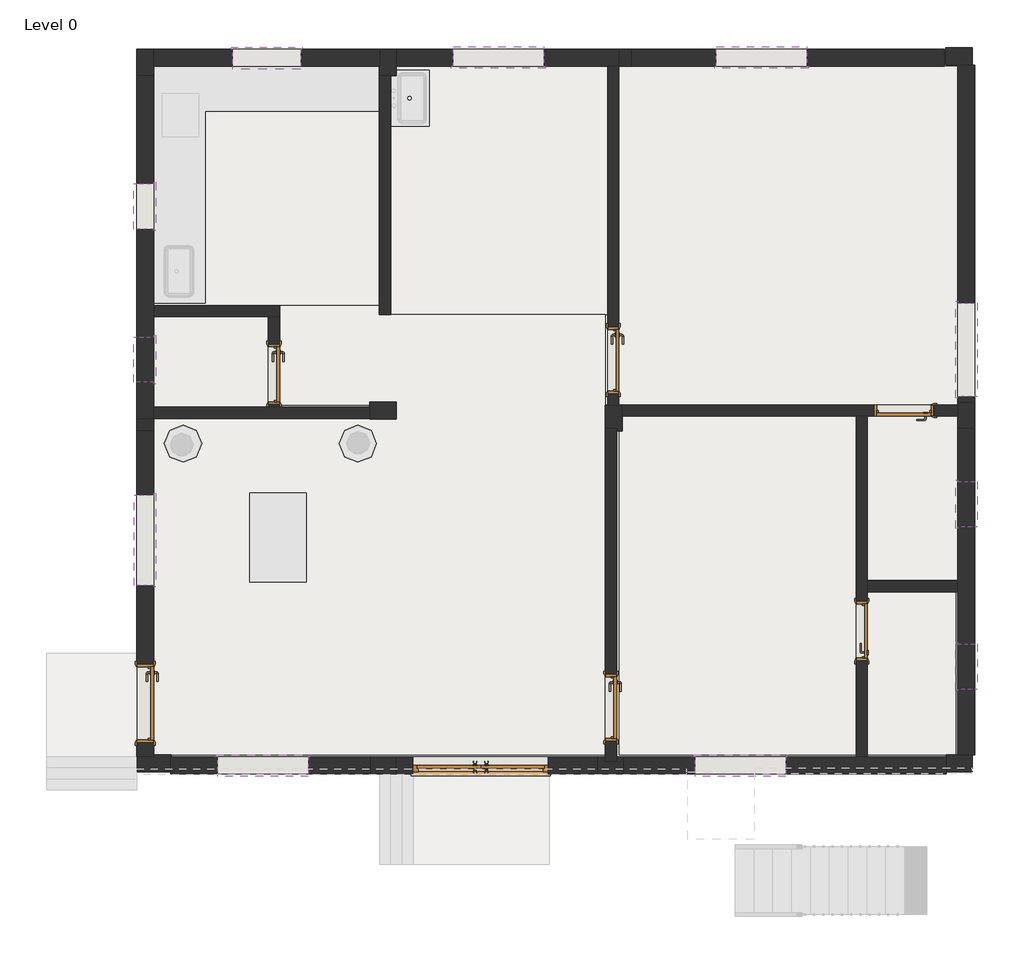
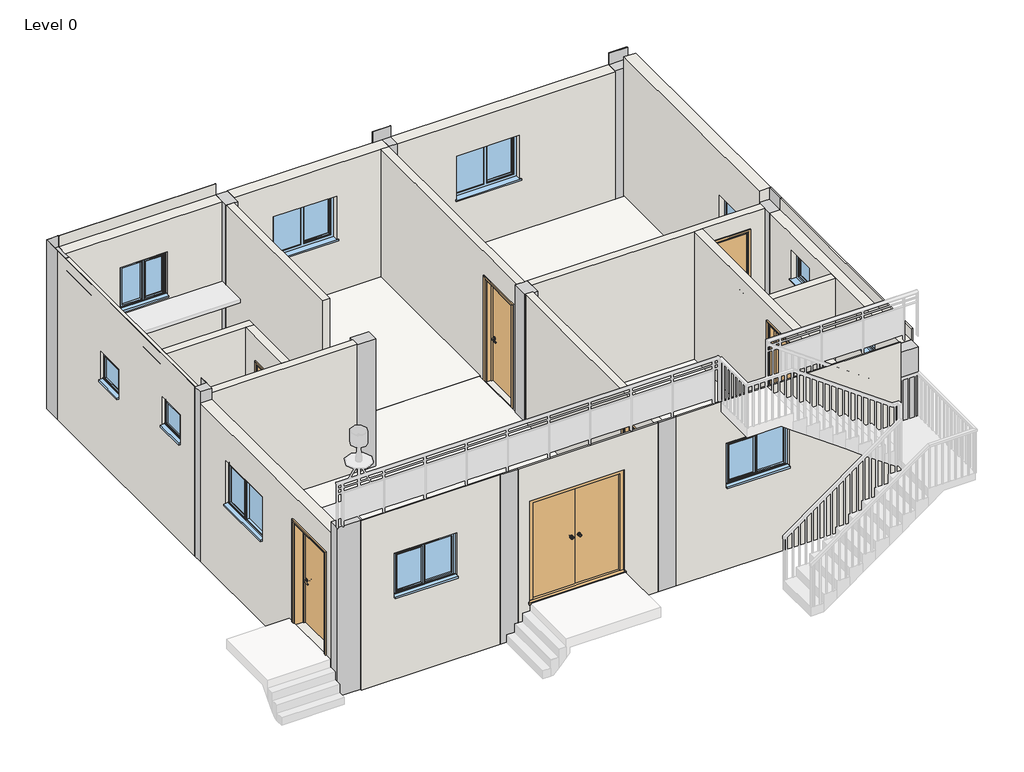
# One storey, part 1 of 3: 19 walls, 12 columns, 11 windows, 7 doors, 5 slabs.
"""IFC4 building model written with IfcOpenShell, lengths in millimetres."""

from ifc_helpers import new_model, si_unit, frame, origin, origin_with_axes, place, context, project, spatial, polyline, outline, extrude, faceted_brep, transform, mapped, element, save
from components import doors_extdbl_flush_d1_7bcd4abb, doors_intsgl_d2_1027b9ee, doors_intsgl_d3_6b78dd6f, doors_intsgl_d4_c85c0d06, doors_intsgl_d5_996c1a6b, doors_intsgl_d7_212e1d6e, windows_dbl_plain_w1_9e0d93ab, windows_dbl_plain_w3_a138f75b, windows_dbl_plain_w5_c0a8d941, windows_dbl_plain_w6_14064f4c, windows_sgl_plain_vw1_399019d4

model = new_model("IFC4")

# Units and contexts
model_context = context("Model", 3, world=origin())
ifc_project = project(units=[si_unit("LENGTHUNIT", "METRE", prefix="MILLI")], contexts=[model_context])

# Site, building, storey
site = spatial("IfcSite", under=ifc_project)
building = spatial("IfcBuilding", under=site)
storey = spatial("IfcBuildingStorey", under=building, Name="Level 0", Elevation=0.0)

# Columns
placement = place(None, origin())
element("IfcColumn", 1, ObjectType="Columns_Rectangular : C1", at=placement, inside=storey, context=model_context, shape_type="Brep", body=[
    faceted_brep([(-10027.7206387, 8256.6134098, 3000.0), (-10256.3206387, 8256.6134098, 3000.0), (-10256.3206387, 7900.9118098, 3000.0), (-10252.3493191, 7900.9118098, 3000.0), (-10252.3493191, 8254.493892, 3000.0), (-10027.7206387, 8254.493892, 3000.0), (-10027.7206387, 8256.6134098, -472.7448), (-10027.7206387, 7900.9118098, -472.7448), (-10256.3206387, 7900.9118098, -472.7448), (-10256.3206387, 8256.6134098, -472.7448), (-10027.7206387, 7900.9118098, 2769.876), (-10252.3493191, 7900.9118098, 2769.876), (-10027.7206387, 8254.493892, 2769.876), (-10252.3493191, 8254.493892, 2769.876)], [[[0, 1, 2, 3, 4, 5]], [[6, 7, 8, 9]], [[1, 0, 6, 9]], [[2, 1, 9, 8]], [[8, 7, 10, 11, 3, 2]], [[7, 6, 0, 5, 12, 10]], [[12, 13, 11, 10]], [[13, 4, 3, 11]], [[4, 13, 12, 5]]]),
])
element("IfcColumn", 2, ObjectType="Columns_Rectangular : C1", at=placement, inside=storey, context=model_context, shape_type="Brep", body=[
    faceted_brep([(-10253.9826298, 3098.473262, 3000.0), (-10025.3826298, 3098.473262, 3000.0), (-10025.3826298, 3454.174862, 3000.0), (-10025.6874298, 3454.174862, 3000.0), (-10025.6874298, 3271.6004551, 3000.0), (-10252.3493191, 3271.6004551, 3000.0), (-10253.9826298, 3271.6004551, 3000.0), (-10025.3826298, 3454.174862, -472.7448), (-10025.3826298, 3098.473262, -472.7448), (-10253.9826298, 3098.473262, -472.7448), (-10253.9826298, 3271.6004551, -472.7448), (-10025.6874298, 3271.6004551, -472.7448), (-10025.6874298, 3454.174862, -472.7448), (-10025.6874298, 3271.6004551, 2769.876)], [[[0, 1, 2, 3, 4, 5, 6]], [[7, 8, 9, 10, 11, 12]], [[2, 7, 12, 3]], [[9, 0, 6, 10]], [[1, 0, 9, 8]], [[2, 1, 8, 7]], [[11, 13, 4, 3, 12]], [[4, 13, 11, 10, 6, 5]]]),
])
element("IfcColumn", 3, ObjectType="Columns_Rectangular : C1", at=placement, inside=storey, context=model_context, shape_type="SweptSolid", body=[
    extrude(outline(polyline([(-6752.3914732, 8254.4587286), (-6752.3914732, 7898.7571286), (-6980.9914732, 7898.7571286), (-6980.9914732, 8026.4804551), (-6975.3482492, 8026.4804551), (-6975.3482492, 8254.4587286), (-6752.3914732, 8254.4587286)])), frame((0.0, 0.0, -472.7448), z_axis=(0.0, 0.0, 1.0), x_axis=(1.0, 0.0, 0.0)), (0.0, 0.0, 1.0), 3242.6208),
])
element("IfcColumn", 4, ObjectType="Columns_Rectangular : C1", at=placement, inside=storey, context=model_context, shape_type="Brep", body=[
    faceted_brep([(-3575.083968, 8257.5084176, 3000.0), (-3930.785568, 8257.5084176, 3000.0), (-3930.785568, 8254.493892, 3000.0), (-3575.083968, 8254.493892, 3000.0), (-3930.785568, 8257.5084176, -472.7448), (-3575.083968, 8257.5084176, -472.7448), (-3575.083968, 8028.9084176, -472.7448), (-3746.8074298, 8028.9084176, -472.7448), (-3746.8074298, 8254.493892, -472.7448), (-3930.785568, 8254.493892, -472.7448), (-3575.083968, 8028.9084176, 2769.876), (-3746.8074298, 8028.9084176, 2769.876), (-3575.083968, 8254.493892, 2769.876), (-3746.8074298, 8254.493892, 2769.876)], [[[0, 1, 2, 3]], [[4, 5, 6, 7, 8, 9]], [[1, 4, 9, 2]], [[7, 6, 10, 11]], [[6, 5, 0, 3, 12, 10]], [[1, 0, 5, 4]], [[9, 8, 13, 12, 3, 2]], [[8, 7, 11, 13]], [[12, 13, 11, 10]]]),
])
element("IfcColumn", 5, ObjectType="Columns_Rectangular : C1", at=placement, inside=storey, context=model_context, shape_type="SweptSolid", body=[
    extrude(outline(polyline([(8277.857647, -472.7448), (8049.257647, -472.7448), (8049.257647, 2769.876), (8254.493892, 2769.876), (8254.493892, 3000.0), (8277.857647, 3000.0), (8277.857647, -472.7448)])), frame((665.5777613, 0.0, 0.0), z_axis=(1.0, 0.0, 0.0), x_axis=(0.0, 1.0, 0.0)), (0.0, 0.0, 1.0), 355.7016),
])
element("IfcColumn", 6, ObjectType="Columns_Rectangular : C1", at=placement, inside=storey, context=model_context, shape_type="Brep", body=[
    faceted_brep([(1055.8403741, 3136.494399, 3000.0), (1055.8403741, 3492.195999, 3000.0), (1025.0682817, 3492.195999, 3000.0), (1025.0682817, 3136.494399, 3000.0), (827.2403741, 3136.494399, -472.7448), (827.2403741, 3492.195999, -472.7448), (1055.8403741, 3492.195999, -472.7448), (1055.8403741, 3136.494399, -472.7448), (1025.0682817, 3136.494399, 2769.876), (827.2403741, 3136.494399, 2769.876), (827.2403741, 3492.195999, 2769.876), (1025.0682817, 3492.195999, 2769.876), (827.2403741, 3301.5242383, 2769.876), (827.2403741, 3453.9242383, 2769.876)], [[[0, 1, 2, 3]], [[4, 5, 6, 7]], [[4, 7, 0, 3, 8, 9]], [[1, 0, 7, 6]], [[6, 5, 10, 11, 2, 1]], [[5, 4, 9, 12, 13, 10]], [[8, 11, 10, 13, 12, 9]], [[11, 8, 3, 2]]]),
])
element("IfcColumn", 7, ObjectType="Columns_Rectangular : C1", at=placement, inside=storey, context=model_context, shape_type="SweptSolid", body=[
    extrude(outline(polyline([(1025.2206817, -1501.142353), (669.5190817, -1501.142353), (669.5190817, -1272.542353), (1025.2206817, -1272.542353), (1025.2206817, -1501.142353)])), frame((0.0, 0.0, -472.7448), z_axis=(0.0, 0.0, 1.0), x_axis=(1.0, 0.0, 0.0)), (0.0, 0.0, 1.0), 3242.6208),
])
element("IfcColumn", 8, ObjectType="Columns_Rectangular : C1", at=placement, inside=storey, context=model_context, shape_type="SweptSolid", body=[
    extrude(outline(polyline([(-7108.0422732, 3492.122462), (-6752.3406732, 3492.122462), (-6752.3406732, 3263.522462), (-7108.0422732, 3263.522462), (-7108.0422732, 3492.122462)])), frame((0.0, 0.0, -472.7448), z_axis=(0.0, 0.0, 1.0), x_axis=(1.0, 0.0, 0.0)), (0.0, 0.0, 1.0), 3242.6208),
])
element("IfcColumn", 9, ObjectType="Columns_Rectangular : C1", at=placement, inside=storey, context=model_context, shape_type="Brep", body=[
    faceted_brep([(-3930.3270396, 3098.192292, -472.7448), (-3930.3270396, 3453.893892, -472.7448), (-3701.7270396, 3453.893892, -472.7448), (-3701.7270396, 3098.192292, -472.7448), (-3701.7270396, 3098.192292, 2769.876), (-3775.2396259, 3098.192292, 2769.876), (-3775.2396259, 3098.192292, 0.0), (-3927.6396259, 3098.192292, 0.0), (-3927.6396259, 3098.192292, 2769.876), (-3930.3270396, 3098.192292, 2769.876), (-3701.7270396, 3453.893892, 2769.876), (-3930.3270396, 3453.893892, 2769.876), (-3927.6396259, 3136.1864821, 2769.876), (-3775.2396259, 3136.1864821, 2769.876), (-3775.2396259, 3136.1864821, 0.0), (-3927.6396259, 3136.1864821, 0.0)], [[[0, 1, 2, 3]], [[0, 3, 4, 5, 6, 7, 8, 9]], [[3, 2, 10, 4]], [[2, 1, 11, 10]], [[1, 0, 9, 11]], [[4, 10, 11, 9, 8, 12, 13, 5]], [[13, 14, 6, 5]], [[15, 12, 8, 7]], [[14, 15, 7, 6]], [[15, 14, 13, 12]]]),
])
element("IfcColumn", 10, ObjectType="Columns_Rectangular : C2", at=placement, inside=storey, context=model_context, shape_type="Brep", body=[
    faceted_brep([(-3680.0785183, -1501.447153, 3000.0), (-4036.4886614, -1501.447153, 3000.0), (-4036.4886614, -1528.9995449, 3000.0), (-3680.0785183, -1528.9995449, 3000.0), (-4036.4886614, -1528.9995449, -472.7448), (-4036.4886614, -1300.3995449, -472.7448), (-3634.7077872, -1300.3995449, -472.7448), (-3634.7077872, -1300.9557617, -472.7448), (-3680.0785183, -1300.9557617, -472.7448), (-3680.0785183, -1528.9995449, -472.7448), (-3634.7077872, -1300.3995449, 2769.876), (-3634.7077872, -1300.9557617, 2769.876), (-4036.4886614, -1300.3995449, 2769.876), (-3927.6396259, -1300.3995449, 2769.876), (-3927.6396259, -1300.3995449, 0.0), (-3775.2396259, -1300.3995449, 0.0), (-3775.2396259, -1300.3995449, 2769.876), (-4036.4886614, -1501.447153, 2769.876), (-3680.0785183, -1501.447153, 2769.876), (-3680.0785183, -1300.9557617, 2769.876), (-3775.2396259, -1359.6135179, 2769.876), (-3927.6396259, -1359.6135179, 2769.876), (-3775.2396259, -1359.6135179, 0.0), (-3927.6396259, -1359.6135179, 0.0)], [[[0, 1, 2, 3]], [[4, 5, 6, 7, 8, 9]], [[6, 10, 11, 7]], [[10, 6, 5, 12, 13, 14, 15, 16]], [[9, 3, 2, 4]], [[17, 12, 5, 4, 2, 1]], [[12, 17, 18, 19, 11, 10, 16, 20, 21, 13]], [[1, 0, 18, 17]], [[9, 8, 19, 18, 0, 3]], [[19, 8, 7, 11]], [[22, 20, 16, 15]], [[21, 23, 14, 13]], [[23, 22, 15, 14]], [[22, 23, 21, 20]]]),
])
element("IfcColumn", 11, ObjectType="Columns_Rectangular : C2", at=placement, inside=storey, context=model_context, shape_type="SweptSolid", body=[
    extrude(outline(polyline([(-1300.3995449, -472.7448), (-1528.9995449, -472.7448), (-1528.9995449, 3000.0), (-1501.447153, 3000.0), (-1501.447153, 2769.876), (-1300.3995449, 2769.876), (-1300.3995449, -472.7448)])), frame((-7102.1088358, 0.0, 0.0), z_axis=(1.0, 0.0, 0.0), x_axis=(0.0, 1.0, 0.0)), (0.0, 0.0, 1.0), 347.8201744),
])
element("IfcColumn", 12, ObjectType="Columns_Rectangular : C2", at=placement, inside=storey, context=model_context, shape_type="Brep", body=[
    faceted_brep([(-10023.7493191, -1272.9298364, 3000.0), (-10023.7493191, -1290.9249414, 3000.0), (-10244.886449, -1290.9249414, 3000.0), (-10244.886449, -1501.5298364, 3000.0), (-9794.5088358, -1501.5298364, 3000.0), (-9794.5088358, -1300.3995449, 3000.0), (-9787.686449, -1300.3995449, 3000.0), (-9787.686449, -1272.9298364, 3000.0), (-10023.7493191, -1290.9249414, -472.7448), (-10023.7493191, -1272.9298364, -472.7448), (-9787.686449, -1272.9298364, -472.7448), (-9787.686449, -1300.3995449, -472.7448), (-9794.5088358, -1300.3995449, -472.7448), (-9794.5088358, -1501.5298364, -472.7448), (-10244.886449, -1501.5298364, -472.7448), (-10244.886449, -1290.9249414, -472.7448), (-10023.7493191, -1290.9249414, 2769.876), (-9794.5088358, -1300.3995449, 2769.876)], [[[0, 1, 2, 3, 4, 5, 6, 7]], [[8, 9, 10, 11, 12, 13, 14, 15]], [[14, 3, 2, 15]], [[3, 14, 13, 4]], [[10, 7, 6, 11]], [[7, 10, 9, 0]], [[8, 16, 1, 0, 9]], [[1, 16, 8, 15, 2]], [[12, 17, 5, 4, 13]], [[5, 17, 12, 11, 6]]]),
])

# Doors
doors_extdbl_flush_d1_shape = doors_extdbl_flush_d1_7bcd4abb(model_context)
element("IfcDoor", 13, ObjectType="Doors_ExtDbl_Flush : D1", at=placement, inside=storey, context=model_context, shape_type="MappedRepresentation", body=[
    mapped(doors_extdbl_flush_d1_shape, transform((-5611.2886614, -1414.6995449, 149.9616), x_axis=(-1.0, 0.0, 0.0), y_axis=(0.0, -1.0, 0.0), z_axis=(0.0, 0.0, 1.0))),
])
doors_intsgl_d2_shape = doors_intsgl_d2_1027b9ee(model_context)
element("IfcDoor", 14, ObjectType="Doors_IntSgl : D2", at=placement, inside=storey, context=model_context, shape_type="MappedRepresentation", body=[
    mapped(doors_intsgl_d2_shape, transform((-10138.0493191, -579.7249414, 149.9616), x_axis=(0.0, -1.0, 0.0), y_axis=(1.0, 0.0, 0.0), z_axis=(0.0, 0.0, 1.0))),
])
doors_intsgl_d3_shape = doors_intsgl_d3_6b78dd6f(model_context)
element("IfcDoor", 15, ObjectType="Doors_IntSgl : D3", at=placement, inside=storey, context=model_context, shape_type="MappedRepresentation", body=[
    mapped(doors_intsgl_d3_shape, transform((-3851.4396259, -635.5438109, 149.9616), x_axis=(0.0, -1.0, 0.0), y_axis=(1.0, 0.0, 0.0), z_axis=(0.0, 0.0, 1.0))),
])
doors_intsgl_d4_shape = doors_intsgl_d4_c85c0d06(model_context)
element("IfcDoor", 16, ObjectType="Doors_IntSgl : D4", at=placement, inside=storey, context=model_context, shape_type="MappedRepresentation", body=[
    mapped(doors_intsgl_d4_shape, transform((-468.1596259, 399.3705356, 304.8), x_axis=(0.0, 1.0, 0.0), y_axis=(-1.0, 0.0, 0.0), z_axis=(0.0, 0.0, 1.0))),
])
doors_intsgl_d5_shape = doors_intsgl_d5_996c1a6b(model_context)
element("IfcDoor", 17, ObjectType="Doors_IntSgl : D5", at=placement, inside=storey, context=model_context, shape_type="MappedRepresentation", body=[
    mapped(doors_intsgl_d5_shape, transform((101.2998395, 3377.7242383, 304.8), x_axis=(-1.0, 0.0, 0.0), y_axis=(0.0, -1.0, 0.0), z_axis=(0.0, 0.0, 1.0))),
])
element("IfcDoor", 18, ObjectType="Doors_IntSgl : D6", at=placement, inside=storey, context=model_context, shape_type="MappedRepresentation", body=[
    mapped(doors_intsgl_d3_shape, transform((-3823.0074298, 4055.6148622, 149.9616), x_axis=(0.0, -1.0, 0.0), y_axis=(1.0, 0.0, 0.0), z_axis=(0.0, 0.0, 1.0))),
])
doors_intsgl_d7_shape = doors_intsgl_d7_212e1d6e(model_context)
element("IfcDoor", 19, ObjectType="Doors_IntSgl : D7", at=placement, inside=storey, context=model_context, shape_type="MappedRepresentation", body=[
    mapped(doors_intsgl_d7_shape, transform((-8401.1034298, 3865.502462, 149.9616), x_axis=(0.0, -1.0, 0.0), y_axis=(1.0, 0.0, 0.0), z_axis=(0.0, 0.0, 1.0))),
])

# Slabs
element("IfcSlab", 20, at=placement, inside=storey, context=model_context, shape_type="SweptSolid", body=[
    extrude(outline(polyline([(-8477.3034298, 4673.086404), (-8477.3034298, 3424.0004551), (-10023.2536634, 3424.0004551), (-10023.2536634, 4673.086404), (-8477.3034298, 4673.086404)])), origin_with_axes(), (0.0, 0.0, 1.0), 149.9616),
])
element("IfcSlab", 21, ObjectType="BEDROOM FLOOR", at=placement, inside=storey, context=model_context, shape_type="SweptSolid", body=[
    extrude(outline(polyline([(825.1925702, 8026.1890784), (825.1925702, 3453.9242383), (-3742.2612698, 3453.9242383), (-3742.2612698, 8026.1890784), (825.1925702, 8026.1890784)])), origin_with_axes(), (0.0, 0.0, 1.0), 149.9616),
    extrude(outline(polyline([(-511.3812698, 3301.7210292), (-511.3812698, -1270.5438109), (-3742.2612698, -1270.5438109), (-3742.2612698, 3301.7210292), (-511.3812698, 3301.7210292)])), origin_with_axes(), (0.0, 0.0, 1.0), 149.9616),
])
element("IfcSlab", 22, ObjectType="KITCHEN FLOOR", at=placement, inside=storey, context=model_context, shape_type="SweptSolid", body=[
    extrude(outline(polyline([(-6975.3482492, 8026.4804551), (-6975.3482492, 4795.6004551), (-10023.2536634, 4795.6004551), (-10023.2536634, 8026.4804551), (-6975.3482492, 8026.4804551)])), origin_with_axes(), (0.0, 0.0, 1.0), 149.9616),
    extrude(outline(polyline([(-3899.2074298, 8026.1890784), (-3899.2074298, 4673.1095286), (-6823.1450401, 4673.1095286), (-6823.1450401, 8026.1890784), (-3899.2074298, 8026.1890784)])), origin_with_axes(), (0.0, 0.0, 1.0), 149.9616),
])
element("IfcSlab", 23, ObjectType="LIVING ROOM", at=placement, inside=storey, context=model_context, shape_type="SweptSolid", body=[
    extrude(outline(polyline([(-10023.2536634, -1270.5438109), (-10023.2536634, 3301.7210292), (-6772.2428349, 3301.7210292), (-6772.2428349, 3453.9095286), (-8347.0428349, 3453.9095286), (-8347.0428349, 4795.6004551), (-6975.4428349, 4795.6004551), (-6975.4428349, 4673.1095286), (-3927.4428349, 4673.1095286), (-3927.4428349, 3301.7210292), (-3927.4428349, -1270.5438109), (-10023.2536634, -1270.5438109)])), origin_with_axes(), (0.0, 0.0, 1.0), 149.9616),
])
element("IfcSlab", 24, ObjectType="TOILET FLOOR", at=placement, inside=storey, context=model_context, shape_type="SweptSolid", body=[
    extrude(outline(polyline([(-422.1369514, 1091.7015114), (-422.1369514, 3301.7210292), (825.1925702, 3301.7210292), (825.1925702, 1091.7015114), (-422.1369514, 1091.7015114)])), frame((0.0, 0.0, 149.9616), z_axis=(0.0, 0.0, 1.0), x_axis=(1.0, 0.0, 0.0)), (0.0, 0.0, 1.0), 149.9616),
    extrude(outline(polyline([(-391.9596259, -1270.5438109), (-391.9596259, 924.0842383), (797.0252143, 924.0842383), (797.0252143, -1270.5438109), (-391.9596259, -1270.5438109)])), frame((0.0, 0.0, 149.9616), z_axis=(0.0, 0.0, 1.0), x_axis=(1.0, 0.0, 0.0)), (0.0, 0.0, 1.0), 149.9616),
])

# Walls
element("IfcWall", 25, ObjectType="EX WALL", at=placement, inside=storey, context=model_context, shape_type="Brep", body=[
    faceted_brep([(-10023.2536634, 8026.4804551, -472.7448), (-6980.9914732, 8026.4804551, -472.7448), (-6975.3482492, 8026.4804551, -472.7448), (-6975.3482492, 8026.4804551, 2769.876), (-6980.9914732, 8026.4804551, 2769.876), (-10023.2536634, 8026.4804551, 2769.876), (-8956.5009563, 8026.4804551, 1200.0), (-8956.5009563, 8026.4804551, 2110.0), (-8042.1009563, 8026.4804551, 2110.0), (-8042.1009563, 8026.4804551, 1200.0), (-6975.3482492, 8255.0804551, -472.7448), (-10023.2536634, 8255.0804551, -472.7448), (-10023.2536634, 8255.0804551, 3000.0), (-6975.3482492, 8255.0804551, 3000.0), (-8956.5009563, 8255.0804551, 2110.0), (-8956.5009563, 8255.0804551, 1200.0), (-8042.1009563, 8255.0804551, 1200.0), (-8042.1009563, 8255.0804551, 2110.0), (-6975.3482492, 8254.4587286, -472.7448), (-6975.3482492, 8254.493892, 3000.0), (-6975.3482492, 8254.493892, 2769.876), (-10023.2536634, 8254.493892, 3000.0), (-10023.2536634, 8254.493892, 2769.876)], [[[0, 1, 2, 3, 4, 5], [6, 7, 8, 9]], [[10, 11, 12, 13], [14, 15, 16, 17]], [[2, 1, 0, 11, 10, 18]], [[10, 13, 19, 20, 3, 2, 18]], [[13, 12, 21, 19]], [[12, 11, 0, 5, 22, 21]], [[15, 14, 7, 6]], [[16, 15, 6, 9]], [[17, 16, 9, 8]], [[14, 17, 8, 7]], [[20, 22, 5, 4, 3]], [[22, 20, 19, 21]]]),
])
element("IfcWall", 26, ObjectType="EX WALL", at=placement, inside=storey, context=model_context, shape_type="Brep", body=[
    faceted_brep([(-6747.0434356, 8025.893892, -472.7448), (-3746.8074298, 8025.893892, -472.7448), (-3746.8074298, 8025.893892, 0.0), (-3746.8074298, 8025.893892, 2769.876), (-3899.2074298, 8025.893892, 2769.876), (-6747.0434356, 8025.893892, 2769.876), (-5985.0434356, 8025.893892, 1200.0), (-5985.0434356, 8025.893892, 2110.0), (-4760.3570356, 8025.893892, 2110.0), (-4760.3570356, 8025.893892, 1200.0), (-3746.8074298, 8254.493892, -472.7448), (-3930.785568, 8254.493892, -472.7448), (-6747.0434356, 8254.493892, -472.7448), (-6747.0434356, 8254.493892, 2769.876), (-3746.8074298, 8254.493892, 2769.876), (-5985.0434356, 8254.493892, 2110.0), (-5985.0434356, 8254.493892, 1200.0), (-4760.3570356, 8254.493892, 1200.0), (-4760.3570356, 8254.493892, 2110.0), (-3746.8074298, 8028.9084176, -472.7448), (-3746.8074298, 8028.9084176, 2769.876)], [[[0, 1, 2, 3, 4, 5], [6, 7, 8, 9]], [[10, 11, 12, 13, 14], [15, 16, 17, 18]], [[1, 0, 12, 11, 10, 19]], [[12, 0, 5, 13]], [[1, 19, 10, 14, 20, 3, 2]], [[16, 15, 7, 6]], [[17, 16, 6, 9]], [[18, 17, 9, 8]], [[15, 18, 8, 7]], [[5, 4, 3, 20, 14, 13]]]),
])
element("IfcWall", 27, ObjectType="EX WALL", at=placement, inside=storey, context=model_context, shape_type="SweptSolid", body=[
    extrude(outline(polyline([(-472.7448, -3572.0383998), (-472.7448, 644.3616002), (2769.876, 644.3616002), (2769.876, -3572.0383998), (-472.7448, -3572.0383998)]), holes=[polyline([(1200.0, -2429.0383998), (2110.0, -2429.0383998), (2110.0, -1209.8383998), (1200.0, -1209.8383998), (1200.0, -2429.0383998)])]), frame((0.0, 8025.893892, 0.0), z_axis=(0.0, 1.0, 0.0), x_axis=(0.0, 0.0, 1.0)), (0.0, 0.0, 1.0), 228.6),
])
element("IfcWall", 28, ObjectType="EX WALL", at=placement, inside=storey, context=model_context, shape_type="SweptSolid", body=[
    extrude(outline(polyline([(8038.8890784, -472.7448), (3492.2890784, -472.7448), (3492.2890784, 3000.0), (8038.8890784, 3000.0), (8038.8890784, -472.7448)]), holes=[polyline([(4829.1418784, 1200.0), (4829.1418784, 2110.0), (3568.4890784, 2110.0), (3568.4890784, 1200.0), (4829.1418784, 1200.0)])]), frame((825.1925702, 0.0, 0.0), z_axis=(1.0, 0.0, 0.0), x_axis=(0.0, 1.0, 0.0)), (0.0, 0.0, 1.0), 228.6),
])
element("IfcWall", 29, ObjectType="EX WALL", at=placement, inside=storey, context=model_context, shape_type="Brep", body=[
    faceted_brep([(827.2403741, 3136.1864821, -472.7448), (827.2403741, -1270.5438109, -472.7448), (827.2403741, -1270.5438109, 2769.876), (827.2403741, 924.0842383, 2769.876), (827.2403741, 1076.4842383, 2769.876), (827.2403741, 3136.1864821, 2769.876), (827.2403741, 2415.5039088, 1828.8), (827.2403741, 2415.5039088, 2438.4), (827.2403741, 1805.9039088, 2438.4), (827.2403741, 1805.9039088, 1828.8), (827.2403741, 221.6213356, 1828.8), (827.2403741, 221.6213356, 2438.4), (827.2403741, -387.9786644, 2438.4), (827.2403741, -387.9786644, 1828.8), (1055.8403741, -1270.5438109, -472.7448), (1055.8403741, 3136.1864821, -472.7448), (1055.8403741, 3136.1864821, 3000.0), (1055.8403741, -1270.5438109, 3000.0), (1055.8403741, 2415.5039088, 2438.4), (1055.8403741, 2415.5039088, 1828.8), (1055.8403741, 1805.9039088, 1828.8), (1055.8403741, 1805.9039088, 2438.4), (1055.8403741, 221.6213356, 2438.4), (1055.8403741, 221.6213356, 1828.8), (1055.8403741, -387.9786644, 1828.8), (1055.8403741, -387.9786644, 2438.4), (1025.0682817, -1270.5438109, 3000.0), (1025.0682817, -1270.5438109, 2769.876), (1025.0682817, 3136.1864821, 3000.0), (1025.0682817, 3136.1864821, 2769.876)], [[[0, 1, 2, 3, 4, 5], [6, 7, 8, 9], [10, 11, 12, 13]], [[14, 15, 16, 17], [18, 19, 20, 21], [22, 23, 24, 25]], [[1, 0, 15, 14]], [[14, 17, 26, 27, 2, 1]], [[17, 16, 28, 26]], [[16, 15, 0, 5, 29, 28]], [[19, 18, 7, 6]], [[20, 19, 6, 9]], [[21, 20, 9, 8]], [[18, 21, 8, 7]], [[23, 22, 11, 10]], [[24, 23, 10, 13]], [[25, 24, 13, 12]], [[22, 25, 12, 11]], [[27, 29, 5, 4, 3, 2]], [[29, 27, 26, 28]]]),
])
element("IfcWall", 30, ObjectType="EX WALL", at=placement, inside=storey, context=model_context, shape_type="Brep", body=[
    faceted_brep([(669.6714817, -1300.9557617, -472.7448), (-3634.7077872, -1300.9557617, -472.7448), (-3680.0785183, -1300.9557617, -472.7448), (-3680.0785183, -1300.9557617, 2769.876), (-3634.7077872, -1300.9557617, 2769.876), (-544.3596259, -1300.9557617, 2769.876), (-391.9596259, -1300.9557617, 2769.876), (669.6714817, -1300.9557617, 2769.876), (-1495.6785183, -1300.9557617, 1200.0), (-1495.6785183, -1300.9557617, 2110.0), (-2714.8785183, -1300.9557617, 2110.0), (-2714.8785183, -1300.9557617, 1200.0), (-3680.0785183, -1529.5557617, -472.7448), (669.6714817, -1529.5557617, -472.7448), (669.6714817, -1529.5557617, 3000.0), (-3680.0785183, -1529.5557617, 3000.0), (-1495.6785183, -1529.5557617, 2110.0), (-1495.6785183, -1529.5557617, 1200.0), (-2714.8785183, -1529.5557617, 1200.0), (-2714.8785183, -1529.5557617, 2110.0), (-3680.0785183, -1528.9995449, -472.7448), (-3680.0785183, -1528.9995449, 3000.0), (-3680.0785183, -1501.447153, 3000.0), (-3680.0785183, -1501.447153, 2769.876), (669.6714817, -1501.447153, 3000.0), (669.6714817, -1501.447153, 2769.876)], [[[0, 1, 2, 3, 4, 5, 6, 7], [8, 9, 10, 11]], [[12, 13, 14, 15], [16, 17, 18, 19]], [[2, 1, 0, 13, 12, 20]], [[12, 15, 21, 22, 23, 3, 2, 20]], [[15, 14, 24, 22, 21]], [[14, 13, 0, 7, 25, 24]], [[17, 16, 9, 8]], [[18, 17, 8, 11]], [[19, 18, 11, 10]], [[16, 19, 10, 9]], [[23, 25, 7, 6, 5, 4, 3]], [[25, 23, 22, 24]]]),
])
element("IfcWall", 31, ObjectType="EX WALL", at=placement, inside=storey, context=model_context, shape_type="Brep", body=[
    faceted_brep([(-4036.4886614, -1300.3995449, -472.7448), (-6754.2886614, -1300.3995449, -472.7448), (-6754.2886614, -1300.3995449, 2769.876), (-4036.4886614, -1300.3995449, 2769.876), (-4696.8886614, -1300.3995449, 149.9616), (-4696.8886614, -1300.3995449, 2259.9616), (-6525.6886614, -1300.3995449, 2259.9616), (-6525.6886614, -1300.3995449, 149.9616), (-6754.2886614, -1528.9995449, -472.7448), (-4036.4886614, -1528.9995449, -472.7448), (-4036.4886614, -1528.9995449, 3000.0), (-6754.2886614, -1528.9995449, 3000.0), (-4696.8886614, -1528.9995449, 2259.9616), (-4696.8886614, -1528.9995449, 149.9616), (-6525.6886614, -1528.9995449, 149.9616), (-6525.6886614, -1528.9995449, 2259.9616), (-6754.2886614, -1501.447153, 3000.0), (-6754.2886614, -1501.447153, 2769.876), (-4036.4886614, -1501.447153, 3000.0), (-4036.4886614, -1501.447153, 2769.876)], [[[0, 1, 2, 3], [4, 5, 6, 7]], [[8, 9, 10, 11], [12, 13, 14, 15]], [[1, 0, 9, 8]], [[8, 11, 16, 17, 2, 1]], [[11, 10, 18, 16]], [[10, 9, 0, 3, 19, 18]], [[13, 12, 5, 4]], [[14, 13, 4, 7]], [[15, 14, 7, 6]], [[12, 15, 6, 5]], [[17, 19, 3, 2]], [[19, 17, 16, 18]]]),
])
element("IfcWall", 32, ObjectType="EX WALL", at=placement, inside=storey, context=model_context, shape_type="Brep", body=[
    faceted_brep([(-7102.1088358, -1300.3995449, -472.7448), (-9787.686449, -1300.3995449, -472.7448), (-9794.5088358, -1300.3995449, -472.7448), (-9794.5088358, -1300.3995449, 2769.876), (-7102.1088358, -1300.3995449, 2769.876), (-7940.3088358, -1300.3995449, 1200.0), (-7940.3088358, -1300.3995449, 2110.0), (-9159.5088358, -1300.3995449, 2110.0), (-9159.5088358, -1300.3995449, 1200.0), (-9794.5088358, -1528.9995449, -472.7448), (-7102.1088358, -1528.9995449, -472.7448), (-7102.1088358, -1528.9995449, 3000.0), (-9794.5088358, -1528.9995449, 3000.0), (-7940.3088358, -1528.9995449, 2110.0), (-7940.3088358, -1528.9995449, 1200.0), (-9159.5088358, -1528.9995449, 1200.0), (-9159.5088358, -1528.9995449, 2110.0), (-9794.5088358, -1501.5298364, -472.7448), (-9794.5088358, -1501.447153, 3000.0), (-9794.5088358, -1501.447153, 2769.876), (-7102.1088358, -1501.447153, 3000.0), (-7102.1088358, -1501.447153, 2769.876)], [[[0, 1, 2, 3, 4], [5, 6, 7, 8]], [[9, 10, 11, 12], [13, 14, 15, 16]], [[2, 1, 0, 10, 9, 17]], [[9, 12, 18, 19, 3, 2, 17]], [[12, 11, 20, 18]], [[11, 10, 0, 4, 21, 20]], [[14, 13, 6, 5]], [[15, 14, 5, 8]], [[16, 15, 8, 7]], [[13, 16, 7, 6]], [[19, 21, 4, 3]], [[21, 19, 18, 20]]]),
])
element("IfcWall", 33, ObjectType="EX WALL", at=placement, inside=storey, context=model_context, shape_type="Brep", body=[
    faceted_brep([(-10023.7493191, -1290.9249414, -472.7448), (-10023.7493191, -1272.9298364, -472.7448), (-10023.7493191, 3098.5198031, -472.7448), (-10023.7493191, 3098.5198031, 2769.876), (-10023.7493191, -1290.9249414, 2769.876), (-10023.7493191, 1015.7198031, 1200.0), (-10023.7493191, 1015.7198031, 2110.0), (-10023.7493191, 2234.9198031, 2110.0), (-10023.7493191, 2234.9198031, 1200.0), (-10023.7493191, -1113.1249414, 149.9616), (-10023.7493191, -1113.1249414, 2259.9616), (-10023.7493191, -46.3249414, 2259.9616), (-10023.7493191, -46.3249414, 149.9616), (-10252.3493191, 3098.5198031, -472.7448), (-10252.3493191, -1290.9249414, -472.7448), (-10252.3493191, -1290.9249414, 2769.876), (-10252.3493191, 3098.5198031, 2769.876), (-10252.3493191, 1015.7198031, 2110.0), (-10252.3493191, 1015.7198031, 1200.0), (-10252.3493191, 2234.9198031, 1200.0), (-10252.3493191, 2234.9198031, 2110.0), (-10252.3493191, -1113.1249414, 2259.9616), (-10252.3493191, -1113.1249414, 149.9616), (-10252.3493191, -46.3249414, 149.9616), (-10252.3493191, -46.3249414, 2259.9616), (-10244.886449, -1290.9249414, -472.7448)], [[[0, 1, 2, 3, 4], [5, 6, 7, 8], [9, 10, 11, 12]], [[13, 14, 15, 16], [17, 18, 19, 20], [21, 22, 23, 24]], [[2, 1, 0, 25, 14, 13]], [[2, 13, 16, 3]], [[14, 25, 0, 4, 15]], [[18, 17, 6, 5]], [[19, 18, 5, 8]], [[20, 19, 8, 7]], [[17, 20, 7, 6]], [[9, 22, 21, 10]], [[10, 21, 24, 11]], [[23, 12, 11, 24]], [[22, 9, 12, 23]], [[4, 3, 16, 15]]]),
])
element("IfcWall", 34, ObjectType="EX WALL", at=placement, inside=storey, context=model_context, shape_type="Brep", body=[
    faceted_brep([(-10025.6874298, 3271.6004551, -472.7448), (-10025.6874298, 3454.174862, -472.7448), (-10025.6874298, 7899.022462, -472.7448), (-10025.6874298, 7899.022462, 2769.876), (-10025.6874298, 3424.0004551, 2769.876), (-10025.6874298, 3271.6004551, 2769.876), (-10025.6874298, 3271.6004551, 0.0), (-10025.6874298, 3758.822462, 1524.0), (-10025.6874298, 3758.822462, 2133.6), (-10025.6874298, 4368.422462, 2133.6), (-10025.6874298, 4368.422462, 1524.0), (-10025.6874298, 5828.922462, 1200.0), (-10025.6874298, 5828.922462, 1809.6), (-10025.6874298, 6438.522462, 1809.6), (-10025.6874298, 6438.522462, 1200.0), (-10254.2874298, 7899.022462, -472.7448), (-10254.2874298, 3271.6004551, -472.7448), (-10254.2874298, 3271.6004551, 3000.0), (-10254.2874298, 7899.022462, 3000.0), (-10254.2874298, 3758.822462, 2133.6), (-10254.2874298, 3758.822462, 1524.0), (-10254.2874298, 4368.422462, 1524.0), (-10254.2874298, 4368.422462, 2133.6), (-10254.2874298, 5828.922462, 1809.6), (-10254.2874298, 5828.922462, 1200.0), (-10254.2874298, 6438.522462, 1200.0), (-10254.2874298, 6438.522462, 1809.6), (-10253.9826298, 3271.6004551, -472.7448), (-10252.3493191, 7899.022462, 3000.0), (-10252.3493191, 7899.022462, 2769.876), (-10253.9826298, 3271.6004551, 3000.0), (-10252.3493191, 3271.6004551, 3000.0), (-10252.3493191, 3271.6004551, 2769.876)], [[[0, 1, 2, 3, 4, 5, 6], [7, 8, 9, 10], [11, 12, 13, 14]], [[15, 16, 17, 18], [19, 20, 21, 22], [23, 24, 25, 26]], [[2, 1, 0, 27, 16, 15]], [[15, 18, 28, 29, 3, 2]], [[18, 17, 30, 31, 28]], [[17, 16, 27, 0, 6, 5, 32, 31, 30]], [[20, 19, 8, 7]], [[21, 20, 7, 10]], [[22, 21, 10, 9]], [[19, 22, 9, 8]], [[24, 23, 12, 11]], [[25, 24, 11, 14]], [[26, 25, 14, 13]], [[23, 26, 13, 12]], [[29, 32, 5, 4, 3]], [[32, 29, 28, 31]]]),
])
element("IfcWall", 35, ObjectType="INNER WALL", at=placement, inside=storey, context=model_context, shape_type="SweptSolid", body=[
    extrude(outline(polyline([(-6977.6874298, 4673.1095286), (-6977.6874298, 7898.9095286), (-6825.2874298, 7898.9095286), (-6825.2874298, 4673.1095286), (-6977.6874298, 4673.1095286)])), origin_with_axes(), (0.0, 0.0, 1.0), 2769.876),
])
element("IfcWall", 36, ObjectType="INNER WALL", at=placement, inside=storey, context=model_context, shape_type="Brep", body=[
    faceted_brep([(-10023.2536634, 4643.2004551, 0.0), (-8477.3034298, 4643.2004551, 0.0), (-8324.9034298, 4643.2004551, 0.0), (-8324.9034298, 4643.2004551, 2769.876), (-8477.3034298, 4643.2004551, 2769.876), (-10023.2536634, 4643.2004551, 2769.876), (-8324.9034298, 4795.6004551, 0.0), (-10023.2536634, 4795.6004551, 0.0), (-10023.2536634, 4795.6004551, 2769.876), (-8324.9034298, 4795.6004551, 2769.876)], [[[0, 1, 2, 3, 4, 5]], [[6, 7, 8, 9]], [[2, 1, 0, 7, 6]], [[7, 0, 5, 8]], [[2, 6, 9, 3]], [[5, 4, 3, 9, 8]]]),
])
element("IfcWall", 37, ObjectType="INNER WALL", at=placement, inside=storey, context=model_context, shape_type="SweptSolid", body=[
    extrude(outline(polyline([(4643.2004551, 0.0), (3424.0004551, 0.0), (3424.0004551, 2769.876), (4643.2004551, 2769.876), (4643.2004551, 0.0)]), holes=[polyline([(3454.022462, 2259.9616), (3454.022462, 149.9616), (4276.982462, 149.9616), (4276.982462, 2259.9616), (3454.022462, 2259.9616)])]), frame((-8477.3034298, 0.0, 0.0), z_axis=(1.0, 0.0, 0.0), x_axis=(0.0, 1.0, 0.0)), (0.0, 0.0, 1.0), 152.4),
])
element("IfcWall", 38, ObjectType="INNER WALL", at=placement, inside=storey, context=model_context, shape_type="Brep", body=[
    faceted_brep([(-10025.6874298, 3271.6004551, 0.0), (-7107.8898732, 3271.6004551, 0.0), (-7107.8898732, 3271.6004551, 2769.876), (-10025.6874298, 3271.6004551, 2769.876), (-7107.8898732, 3424.0004551, 0.0), (-8324.9034298, 3424.0004551, 0.0), (-8477.3034298, 3424.0004551, 0.0), (-10025.6874298, 3424.0004551, 0.0), (-10025.6874298, 3424.0004551, 2769.876), (-8477.3034298, 3424.0004551, 2769.876), (-8324.9034298, 3424.0004551, 2769.876), (-7107.8898732, 3424.0004551, 2769.876)], [[[0, 1, 2, 3]], [[4, 5, 6, 7, 8, 9, 10, 11]], [[1, 0, 7, 6, 5, 4]], [[1, 4, 11, 2]], [[7, 0, 3, 8]], [[3, 2, 11, 10, 9, 8]]]),
])
element("IfcWall", 39, ObjectType="INNER WALL", at=placement, inside=storey, context=model_context, shape_type="SweptSolid", body=[
    extrude(outline(polyline([(8025.893892, 0.0), (3453.9242383, 0.0), (3453.9242383, 2769.876), (8025.893892, 2769.876), (8025.893892, 0.0)]), holes=[polyline([(3598.4148622, 2259.9616), (3598.4148622, 149.9616), (4512.8148622, 149.9616), (4512.8148622, 2259.9616), (3598.4148622, 2259.9616)])]), frame((-3899.2074298, 0.0, 0.0), z_axis=(1.0, 0.0, 0.0), x_axis=(0.0, 1.0, 0.0)), (0.0, 0.0, 1.0), 152.4),
])
element("IfcWall", 40, ObjectType="INNER WALL", at=placement, inside=storey, context=model_context, shape_type="Brep", body=[
    faceted_brep([(-3699.1380213, 3301.5242383, 0.0), (-544.3596259, 3301.5242383, 0.0), (-391.9596259, 3301.5242383, 0.0), (827.2403741, 3301.5242383, 0.0), (827.2403741, 3301.5242383, 2769.876), (-391.9596259, 3301.5242383, 2769.876), (-544.3596259, 3301.5242383, 2769.876), (-3699.1380213, 3301.5242383, 2769.876), (-305.1509605, 3301.5242383, 304.8), (-305.1509605, 3301.5242383, 2414.8), (507.7506395, 3301.5242383, 2414.8), (507.7506395, 3301.5242383, 304.8), (827.2403741, 3453.9242383, 0.0), (-3699.1380213, 3453.9242383, 0.0), (-3699.1380213, 3453.9242383, 2769.876), (827.2403741, 3453.9242383, 2769.876), (-305.1509605, 3453.9242383, 2414.8), (-305.1509605, 3453.9242383, 304.8), (507.7506395, 3453.9242383, 304.8), (507.7506395, 3453.9242383, 2414.8)], [[[0, 1, 2, 3, 4, 5, 6, 7], [8, 9, 10, 11]], [[12, 13, 14, 15], [16, 17, 18, 19]], [[3, 2, 1, 0, 13, 12]], [[3, 12, 15, 4]], [[13, 0, 7, 14]], [[8, 17, 16, 9]], [[9, 16, 19, 10]], [[18, 11, 10, 19]], [[17, 8, 11, 18]], [[7, 6, 5, 4, 15, 14]]]),
])
element("IfcWall", 41, ObjectType="INNER WALL", at=placement, inside=storey, context=model_context, shape_type="Brep", body=[
    faceted_brep([(-544.3596259, 3301.5242383, 0.0), (-544.3596259, -1300.9557617, 0.0), (-544.3596259, -1300.9557617, 2769.876), (-544.3596259, 3301.5242383, 2769.876), (-544.3596259, 805.8213356, 304.8), (-544.3596259, 805.8213356, 2414.8), (-544.3596259, -7.0802644, 2414.8), (-544.3596259, -7.0802644, 304.8), (-391.9596259, -1300.9557617, 0.0), (-391.9596259, 924.0842383, 0.0), (-391.9596259, 1076.4842383, 0.0), (-391.9596259, 3301.5242383, 0.0), (-391.9596259, 3301.5242383, 2769.876), (-391.9596259, 1076.4842383, 2769.876), (-391.9596259, 924.0842383, 2769.876), (-391.9596259, -1300.9557617, 2769.876), (-391.9596259, 805.8213356, 2414.8), (-391.9596259, 805.8213356, 304.8), (-391.9596259, -7.0802644, 304.8), (-391.9596259, -7.0802644, 2414.8)], [[[0, 1, 2, 3], [4, 5, 6, 7]], [[8, 9, 10, 11, 12, 13, 14, 15], [16, 17, 18, 19]], [[1, 0, 11, 10, 9, 8]], [[11, 0, 3, 12]], [[4, 17, 16, 5]], [[5, 16, 19, 6]], [[18, 7, 6, 19]], [[17, 4, 7, 18]], [[3, 2, 15, 14, 13, 12]], [[1, 8, 15, 2]]]),
])
element("IfcWall", 42, ObjectType="INNER WALL", at=placement, inside=storey, context=model_context, shape_type="SweptSolid", body=[
    extrude(outline(polyline([(-391.9596259, 1076.4842383), (827.2403741, 1076.4842383), (827.2403741, 924.0842383), (-391.9596259, 924.0842383), (-391.9596259, 1076.4842383)])), origin_with_axes(), (0.0, 0.0, 1.0), 2769.876),
])
element("IfcWall", 43, ObjectType="INNER WALL", at=placement, inside=storey, context=model_context, shape_type="Brep", body=[
    faceted_brep([(-3775.2396259, -1359.6135179, 0.0), (-3775.2396259, -1300.3995449, 0.0), (-3775.2396259, 3098.192292, 0.0), (-3775.2396259, 3136.1864821, 0.0), (-3775.2396259, 3136.1864821, 2769.876), (-3775.2396259, 3098.192292, 2769.876), (-3775.2396259, -1300.3995449, 2769.876), (-3775.2396259, -1359.6135179, 2769.876), (-3775.2396259, -1092.7438109, 149.9616), (-3775.2396259, -1092.7438109, 2259.9616), (-3775.2396259, -178.3438109, 2259.9616), (-3775.2396259, -178.3438109, 149.9616), (-3927.6396259, 3136.1864821, 0.0), (-3927.6396259, 3098.192292, 0.0), (-3927.6396259, -1300.3995449, 0.0), (-3927.6396259, -1359.6135179, 0.0), (-3927.6396259, -1359.6135179, 2769.876), (-3927.6396259, -1300.3995449, 2769.876), (-3927.6396259, 3098.192292, 2769.876), (-3927.6396259, 3136.1864821, 2769.876), (-3927.6396259, -1092.7438109, 2259.9616), (-3927.6396259, -1092.7438109, 149.9616), (-3927.6396259, -178.3438109, 149.9616), (-3927.6396259, -178.3438109, 2259.9616)], [[[0, 1, 2, 3, 4, 5, 6, 7], [8, 9, 10, 11]], [[12, 13, 14, 15, 16, 17, 18, 19], [20, 21, 22, 23]], [[3, 2, 1, 0, 15, 14, 13, 12]], [[3, 12, 19, 4]], [[15, 0, 7, 16]], [[8, 21, 20, 9]], [[9, 20, 23, 10]], [[22, 11, 10, 23]], [[21, 8, 11, 22]], [[7, 6, 5, 4, 19, 18, 17, 16]]]),
])

# Windows
windows_dbl_plain_w1_shape = windows_dbl_plain_w1_9e0d93ab(model_context)
element("IfcWindow", 44, ObjectType="Windows_Dbl_Plain : W1", at=placement, inside=storey, context=model_context, shape_type="MappedRepresentation", body=[
    mapped(windows_dbl_plain_w1_shape, transform((-8834.9088358, -1406.2429771, 0.0), x_axis=(-1.0, 0.0, 0.0), y_axis=(0.0, -1.0, 0.0), z_axis=(0.0, 0.0, 1.0))),
])
windows_dbl_plain_w3_shape = windows_dbl_plain_w3_a138f75b(model_context)
element("IfcWindow", 45, ObjectType="Windows_Dbl_Plain : W3", at=placement, inside=storey, context=model_context, shape_type="MappedRepresentation", body=[
    mapped(windows_dbl_plain_w3_shape, transform((931.0360023, 3913.8154784, 0.0), x_axis=(0.0, -1.0, 0.0), y_axis=(1.0, 0.0, 0.0), z_axis=(0.0, 0.0, 1.0))),
])
element("IfcWindow", 46, ObjectType="Windows_Dbl_Plain : W4", at=placement, inside=storey, context=model_context, shape_type="MappedRepresentation", body=[
    mapped(windows_dbl_plain_w1_shape, transform((-1534.4383998, 8131.7373242, 0.0), x_axis=(1.0, 0.0, 0.0), y_axis=(0.0, 1.0, 0.0), z_axis=(0.0, 0.0, 1.0))),
])
windows_dbl_plain_w5_shape = windows_dbl_plain_w5_c0a8d941(model_context)
element("IfcWindow", 47, ObjectType="Windows_Dbl_Plain : W5", at=placement, inside=storey, context=model_context, shape_type="MappedRepresentation", body=[
    mapped(windows_dbl_plain_w5_shape, transform((-5087.7002356, 8131.7373242, 0.0), x_axis=(1.0, 0.0, 0.0), y_axis=(0.0, 1.0, 0.0), z_axis=(0.0, 0.0, 1.0))),
])
windows_dbl_plain_w6_shape = windows_dbl_plain_w6_14064f4c(model_context)
element("IfcWindow", 48, ObjectType="Windows_Dbl_Plain : W6", at=placement, inside=storey, context=model_context, shape_type="MappedRepresentation", body=[
    mapped(windows_dbl_plain_w6_shape, transform((-8214.3009563, 8149.2370229, 0.0), x_axis=(1.0, 0.0, 0.0), y_axis=(0.0, 1.0, 0.0), z_axis=(0.0, 0.0, 1.0))),
])
element("IfcWindow", 49, ObjectType="Windows_Dbl_Plain : W7", at=placement, inside=storey, context=model_context, shape_type="MappedRepresentation", body=[
    mapped(windows_dbl_plain_w1_shape, transform((-10129.5927513, 1910.3198031, 0.0), x_axis=(0.0, 1.0, 0.0), y_axis=(-1.0, 0.0, 0.0), z_axis=(0.0, 0.0, 1.0))),
])
element("IfcWindow", 50, ObjectType="Windows_Dbl_Plain : WN", at=placement, inside=storey, context=model_context, shape_type="MappedRepresentation", body=[
    mapped(windows_dbl_plain_w1_shape, transform((-2390.2785183, -1406.7991939, 0.0), x_axis=(-1.0, 0.0, 0.0), y_axis=(0.0, -1.0, 0.0), z_axis=(0.0, 0.0, 1.0))),
])
windows_sgl_plain_vw1_shape = windows_sgl_plain_vw1_399019d4(model_context)
element("IfcWindow", 51, ObjectType="Windows_Sgl_Plain : VW1", at=placement, inside=storey, context=model_context, shape_type="MappedRepresentation", body=[
    mapped(windows_sgl_plain_vw1_shape, transform((-10131.530862, 4063.622462, 23.6), x_axis=(0.0, 1.0, 0.0), y_axis=(-1.0, 0.0, 0.0), z_axis=(0.0, 0.0, 1.0))),
])
element("IfcWindow", 52, ObjectType="Windows_Sgl_Plain : VW2", at=placement, inside=storey, context=model_context, shape_type="MappedRepresentation", body=[
    mapped(windows_sgl_plain_vw1_shape, transform((-10131.530862, 6133.722462, -300.4), x_axis=(0.0, 1.0, 0.0), y_axis=(-1.0, 0.0, 0.0), z_axis=(0.0, 0.0, 1.0))),
])
element("IfcWindow", 53, ObjectType="Windows_Sgl_Plain : VW3", at=placement, inside=storey, context=model_context, shape_type="MappedRepresentation", body=[
    mapped(windows_sgl_plain_vw1_shape, transform((933.0838063, 2110.7039088, 328.4), x_axis=(0.0, -1.0, 0.0), y_axis=(1.0, 0.0, 0.0), z_axis=(0.0, 0.0, 1.0))),
])
element("IfcWindow", 54, ObjectType="Windows_Sgl_Plain : VW4", at=placement, inside=storey, context=model_context, shape_type="MappedRepresentation", body=[
    mapped(windows_sgl_plain_vw1_shape, transform((933.0838063, -83.1786644, 328.4), x_axis=(0.0, -1.0, 0.0), y_axis=(1.0, 0.0, 0.0), z_axis=(0.0, 0.0, 1.0))),
])

save(model, "model.ifc")

# Revit data of these elements
# Type "Columns_Rectangular : C1"
#   Keynote = "G"
#   Depth = 1.167 ft
#   Offset Base = 0.0 ft
#   Offset Top = 0.0 ft
#   Width = 0.75 ft
#   Material = Concrete, Precast
# Type "Columns_Rectangular : C2"
#   Keynote = "G"
#   Depth = 1.5 ft
#   Offset Base = 0.0 ft
#   Offset Top = 0.0 ft
#   Width = 0.75 ft
#   Material = Concrete, Precast
# Type "Doors_ExtDbl_Flush : D1"
#   Type Mark = "52"
#   Type Comments = "External Double"
#   Operation = "DoubleDoorSingleSwing"
#   Keynote = "L20"
#   Analytic Construction = "Metal"
#   Wrap Layers (Ext) from Ext = 0.336286 ft
#   Wrap Layers (Int) from Ext = 0.582349 ft
#   Thickness = 0.144357 ft
#   Rough Width = 6.0 ft
#   Rough Height = 6.922572 ft
#   O/A Frame Width = 0.209974 ft
#   Heat Transfer Coefficient (U) = 3.7021 W/(m²·K)
#   Handle Z Distance = 3.444882 ft
#   FrameWidth = 0.137795 ft
#   FrameOffset - External = 0.082021 ft
#   FrameDepth = 0.291995 ft
#   Door Panel Width = 2.826115 ft
#   Door Panel Thickness = 0.144357 ft
#   Door Panel Height = 6.56168 ft
#   Cill Thickness = 0.178806 ft
#   Cill Projection = 0.098425 ft
#   Handle X Distance = 0.246063 ft
#   Height = 6.922572 ft
#   Structural Tolerance = 0.021325 ft
#   Tolerance = 0.009843 ft
#   Undercut = 0.013123 ft
#   Width = 6.0 ft
#   Cill Extension = 0.082021 ft
#   Cavity Closer Width = 0.164042 ft
#   Cavity Closer Offset from Ext = 0.336286 ft
#   Cavity Closer Depth = 0.278871 ft
#   Vis - Ironmongery = yes
#   Vis - Cavity Closers = yes
#   Function = 1
#   Material Door = Door - Panel
#   Material Frame = Door - Frame/Mullion
#   Material Ironmongery = Door - Handle
#   Visual Light Transmittance = 0
#   Thermal Resistance (R) = 0
#   Solar Heat Gain Coefficient = 0
#   Wall Closure = (empty or 0)
# Type "Doors_IntSgl : D2"
#   Type Mark = "49"
#   Type Comments = "Internal Single"
#   Operation = "SingleSwingRight"
#   Manufacturer = "Revit"
#   Keynote = "L20"
#   Description = "Internal Single Door"
#   Analytic Construction = "Metal"
#   UnderCut = 0.026247 ft
#   Tolerance = 0.006562 ft
#   Thickness = 0.124672 ft
#   Thermal Resistance (R) = 0.270117 (m²·K)/W
#   Structural Tolerance = 0.026247 ft
#   StopDepth = 0.104987 ft
#   Stop Thickness = 0.062336 ft
#   Rough Width = 3.5 ft
#   Rough Height = 6.922572 ft
#   Height to Top Lock Rail = 3.28084 ft
#   Heat Transfer Coefficient (U) = 3.7021 W/(m²·K)
#   Handle Z Distance = 2.952756 ft
#   Handle X Distance = 0.246063 ft
#   Frame Thickness = 0.104987 ft
#   Door Panel Width = 3.224409 ft
#   Door Panel Thickness = 0.124672 ft
#   Door Panel Offset = 0.0 ft
#   Height = 6.922572 ft
#   Width = 3.5 ft
#   Door Panel Height = 6.75853 ft
#   Architrave Setback = 0.016404 ft
#   Vis - Ironmongery = yes
#   Material Ironmongery = Door - Handle
#   Material Frame = Door - Frame/Mullion (1)
#   Material Door = Door - Panel
#   Material Architrave = Door - Architrave
#   Visual Light Transmittance = 0
#   Solar Heat Gain Coefficient = 0
#   Function = (empty or 0)
#   Wall Closure = (empty or 0)
# Type "Doors_IntSgl : D3"
#   Type Mark = "51"
#   Type Comments = "Internal Single"
#   Operation = "SingleSwingRight"
#   Manufacturer = "Revit"
#   Keynote = "L20"
#   Description = "Internal Single Door"
#   Analytic Construction = "Metal"
#   UnderCut = 0.026247 ft
#   Tolerance = 0.006562 ft
#   Thickness = 0.124672 ft
#   Thermal Resistance (R) = 0.270117 (m²·K)/W
#   Structural Tolerance = 0.026247 ft
#   StopDepth = 0.104987 ft
#   Stop Thickness = 0.062336 ft
#   Rough Width = 3.0 ft
#   Rough Height = 6.922572 ft
#   Height to Top Lock Rail = 3.28084 ft
#   Heat Transfer Coefficient (U) = 3.7021 W/(m²·K)
#   Handle Z Distance = 2.952756 ft
#   Handle X Distance = 0.246063 ft
#   Frame Thickness = 0.104987 ft
#   Door Panel Width = 2.724409 ft
#   Door Panel Thickness = 0.124672 ft
#   Door Panel Offset = 0.0 ft
#   Height = 6.922572 ft
#   Width = 3.0 ft
#   Door Panel Height = 6.75853 ft
#   Architrave Setback = 0.016404 ft
#   Vis - Ironmongery = yes
#   Material Ironmongery = Door - Handle
#   Material Frame = Door - Frame/Mullion (1)
#   Material Door = Door - Panel
#   Material Architrave = Door - Architrave
#   Visual Light Transmittance = 0
#   Solar Heat Gain Coefficient = 0
#   Function = (empty or 0)
#   Wall Closure = (empty or 0)
# Type "Doors_IntSgl : D4"
#   Type Mark = "50"
#   Type Comments = "Internal Single"
#   Operation = "SingleSwingRight"
#   Manufacturer = "Revit"
#   Keynote = "L20"
#   Description = "Internal Single Door"
#   Analytic Construction = "Metal"
#   UnderCut = 0.026247 ft
#   Tolerance = 0.006562 ft
#   Thickness = 0.124672 ft
#   Thermal Resistance (R) = 0.270117 (m²·K)/W
#   Structural Tolerance = 0.026247 ft
#   StopDepth = 0.104987 ft
#   Stop Thickness = 0.062336 ft
#   Rough Width = 2.667 ft
#   Rough Height = 6.922572 ft
#   Height to Top Lock Rail = 3.28084 ft
#   Heat Transfer Coefficient (U) = 3.7021 W/(m²·K)
#   Handle Z Distance = 2.952756 ft
#   Handle X Distance = 0.246063 ft
#   Frame Thickness = 0.104987 ft
#   Door Panel Width = 2.391409 ft
#   Door Panel Thickness = 0.124672 ft
#   Door Panel Offset = 0.0 ft
#   Height = 6.922572 ft
#   Width = 2.667 ft
#   Door Panel Height = 6.75853 ft
#   Architrave Setback = 0.016404 ft
#   Vis - Ironmongery = yes
#   Material Ironmongery = Door - Handle
#   Material Frame = Door - Frame/Mullion (1)
#   Material Door = Door - Panel
#   Material Architrave = Door - Architrave
#   Visual Light Transmittance = 0
#   Solar Heat Gain Coefficient = 0
#   Function = (empty or 0)
#   Wall Closure = (empty or 0)
# Type "Doors_IntSgl : D5"
#   Type Mark = "48"
#   Type Comments = "Internal Single"
#   Operation = "SingleSwingRight"
#   Manufacturer = "Revit"
#   Keynote = "L20"
#   Description = "Internal Single Door"
#   Analytic Construction = "Metal"
#   UnderCut = 0.026247 ft
#   Tolerance = 0.006562 ft
#   Thickness = 0.124672 ft
#   Thermal Resistance (R) = 0.270117 (m²·K)/W
#   Structural Tolerance = 0.026247 ft
#   StopDepth = 0.104987 ft
#   Stop Thickness = 0.062336 ft
#   Rough Width = 2.667 ft
#   Rough Height = 6.922572 ft
#   Height to Top Lock Rail = 3.28084 ft
#   Heat Transfer Coefficient (U) = 3.7021 W/(m²·K)
#   Handle Z Distance = 2.952756 ft
#   Handle X Distance = 0.246063 ft
#   Frame Thickness = 0.104987 ft
#   Door Panel Width = 2.391409 ft
#   Door Panel Thickness = 0.124672 ft
#   Door Panel Offset = 0.0 ft
#   Height = 6.922572 ft
#   Width = 2.667 ft
#   Door Panel Height = 6.75853 ft
#   Architrave Setback = 0.016404 ft
#   Vis - Ironmongery = yes
#   Material Ironmongery = Door - Handle
#   Material Frame = Door - Frame/Mullion (1)
#   Material Door = Door - Panel
#   Material Architrave = Door - Architrave
#   Visual Light Transmittance = 0
#   Solar Heat Gain Coefficient = 0
#   Function = (empty or 0)
#   Wall Closure = (empty or 0)
# Type "Doors_IntSgl : D6"
#   Type Mark = "47"
#   Type Comments = "Internal Single"
#   Operation = "SingleSwingRight"
#   Manufacturer = "Revit"
#   Keynote = "L20"
#   Description = "Internal Single Door"
#   Analytic Construction = "Metal"
#   UnderCut = 0.026247 ft
#   Tolerance = 0.006562 ft
#   Thickness = 0.124672 ft
#   Thermal Resistance (R) = 0.270117 (m²·K)/W
#   Structural Tolerance = 0.026247 ft
#   StopDepth = 0.104987 ft
#   Stop Thickness = 0.062336 ft
#   Rough Width = 3.0 ft
#   Rough Height = 6.922572 ft
#   Height to Top Lock Rail = 3.28084 ft
#   Heat Transfer Coefficient (U) = 3.7021 W/(m²·K)
#   Handle Z Distance = 2.952756 ft
#   Handle X Distance = 0.246063 ft
#   Frame Thickness = 0.104987 ft
#   Door Panel Width = 2.724409 ft
#   Door Panel Thickness = 0.124672 ft
#   Door Panel Offset = 0.0 ft
#   Height = 6.922572 ft
#   Width = 3.0 ft
#   Door Panel Height = 6.75853 ft
#   Architrave Setback = 0.016404 ft
#   Vis - Ironmongery = yes
#   Material Ironmongery = Door - Handle
#   Material Frame = Door - Frame/Mullion (1)
#   Material Door = Door - Panel
#   Material Architrave = Door - Architrave
#   Visual Light Transmittance = 0
#   Solar Heat Gain Coefficient = 0
#   Function = (empty or 0)
#   Wall Closure = (empty or 0)
# Type "Doors_IntSgl : D7"
#   Type Mark = "46"
#   Type Comments = "Internal Single"
#   Operation = "SingleSwingRight"
#   Manufacturer = "Revit"
#   Keynote = "L20"
#   Description = "Internal Single Door"
#   Analytic Construction = "Metal"
#   UnderCut = 0.026247 ft
#   Tolerance = 0.006562 ft
#   Thickness = 0.124672 ft
#   Thermal Resistance (R) = 0.270117 (m²·K)/W
#   Structural Tolerance = 0.026247 ft
#   StopDepth = 0.104987 ft
#   Stop Thickness = 0.062336 ft
#   Rough Width = 2.7 ft
#   Rough Height = 6.922572 ft
#   Height to Top Lock Rail = 3.28084 ft
#   Heat Transfer Coefficient (U) = 3.7021 W/(m²·K)
#   Handle Z Distance = 2.952756 ft
#   Handle X Distance = 0.246063 ft
#   Frame Thickness = 0.104987 ft
#   Door Panel Width = 2.424409 ft
#   Door Panel Thickness = 0.124672 ft
#   Door Panel Offset = 0.0 ft
#   Height = 6.922572 ft
#   Width = 2.7 ft
#   Door Panel Height = 6.75853 ft
#   Architrave Setback = 0.016404 ft
#   Vis - Ironmongery = yes
#   Material Ironmongery = Door - Handle
#   Material Frame = Door - Frame/Mullion (1)
#   Material Door = Door - Panel
#   Material Architrave = Door - Architrave
#   Visual Light Transmittance = 0
#   Solar Heat Gain Coefficient = 0
#   Function = (empty or 0)
#   Wall Closure = (empty or 0)
# Type
#   Function = 0
# Type "BEDROOM FLOOR"
#   Function = 0
#   Layers, outside or top first: 0.072 ft "BEDROOM FLOOR TEXTURE" (function 5); 0.42 ft "Structure, Timber Joist/Rafter Layer" (function 1)
# Type "KITCHEN FLOOR"
#   Function = 0
#   Layers, outside or top first: 0.072 ft "KITCHEN FLOOR TEXTURE" (function 5); 0.42 ft "Structure, Timber Joist/Rafter Layer" (function 1)
# Type "LIVING ROOM"
#   Function = 0
#   Layers, outside or top first: 0.072 ft "LIVING ROOM FLOOR TEXTURE" (function 5); 0.42 ft "Structure, Timber Joist/Rafter Layer" (function 1)
# Type "TOILET FLOOR"
#   Function = 0
#   Layers, outside or top first: 0.072 ft "TOILET FLOOR TEXTURE" (function 5); 0.42 ft "Structure, Timber Joist/Rafter Layer" (function 1)
# Type "EX WALL"
#   Keynote = "F10"
#   Layers, outside or top first: 0.75 ft "Brick, Common" (function 1)
# Type "INNER WALL"
#   Keynote = "F10"
#   Layers, outside or top first: 0.5 ft "Brick, Common" (function 1)
# Type "Windows_Dbl_Plain : W1"
#   Type Mark = "62"
#   Operation = "DoublePanelVertical"
#   Construction Type Id = "GSP4R"
#   Manufacturer = "Revit"
#   Keynote = "L10"
#   Analytic Construction = "1/8 in Pilkington single glazing"
#   Wrap Layers (Ext) from Ext = 0.336286 ft
#   Wrap Layers (Int) from Ext = 0.582349 ft
#   Window Board Projection = 0.082021 ft
#   Window Board Extension = 0.082021 ft
#   Visual Light Transmittance = 0.9
#   Solar Heat Gain Coefficient = 0.78
#   Rough Width = 4.0 ft
#   Rough Height = 2.985564 ft
#   Height = 2.985564 ft
#   Width = 4.0 ft
#   Heat Transfer Coefficient (U) = 3.6886 W/(m²·K)
#   Glazing Thickness = 0.07874 ft
#   FrameOffset - External = 0.164042 ft
#   Frame Depth = 0.213255 ft
#   Default Head Height = 6.922572 ft
#   Cill Depth = 0.287073 ft
#   Cavity Closer Width = 0.164042 ft
#   Cavity Closer Offset from Ext = 0.336286 ft
#   Cavity Closer Depth = 0.278871 ft
#   Vis - Cavity Closers = yes
#   Define Thermal Properties by = 1
#   Material Trim = Window Frame
#   Material Glass = Glass
#   Material Frame = Cherry
#   Wall Closure = (empty or 0)
# Type "Windows_Dbl_Plain : W3"
#   Type Mark = "59"
#   Operation = "DoublePanelVertical"
#   Construction Type Id = "GSP4R"
#   Manufacturer = "Revit"
#   Keynote = "L10"
#   Analytic Construction = "1/8 in Pilkington single glazing"
#   Wrap Layers (Ext) from Ext = 0.336286 ft
#   Wrap Layers (Int) from Ext = 0.582349 ft
#   Window Board Projection = 0.082021 ft
#   Window Board Extension = 0.082021 ft
#   Visual Light Transmittance = 0.9
#   Solar Heat Gain Coefficient = 0.78
#   Rough Width = 4.136 ft
#   Rough Height = 2.985564 ft
